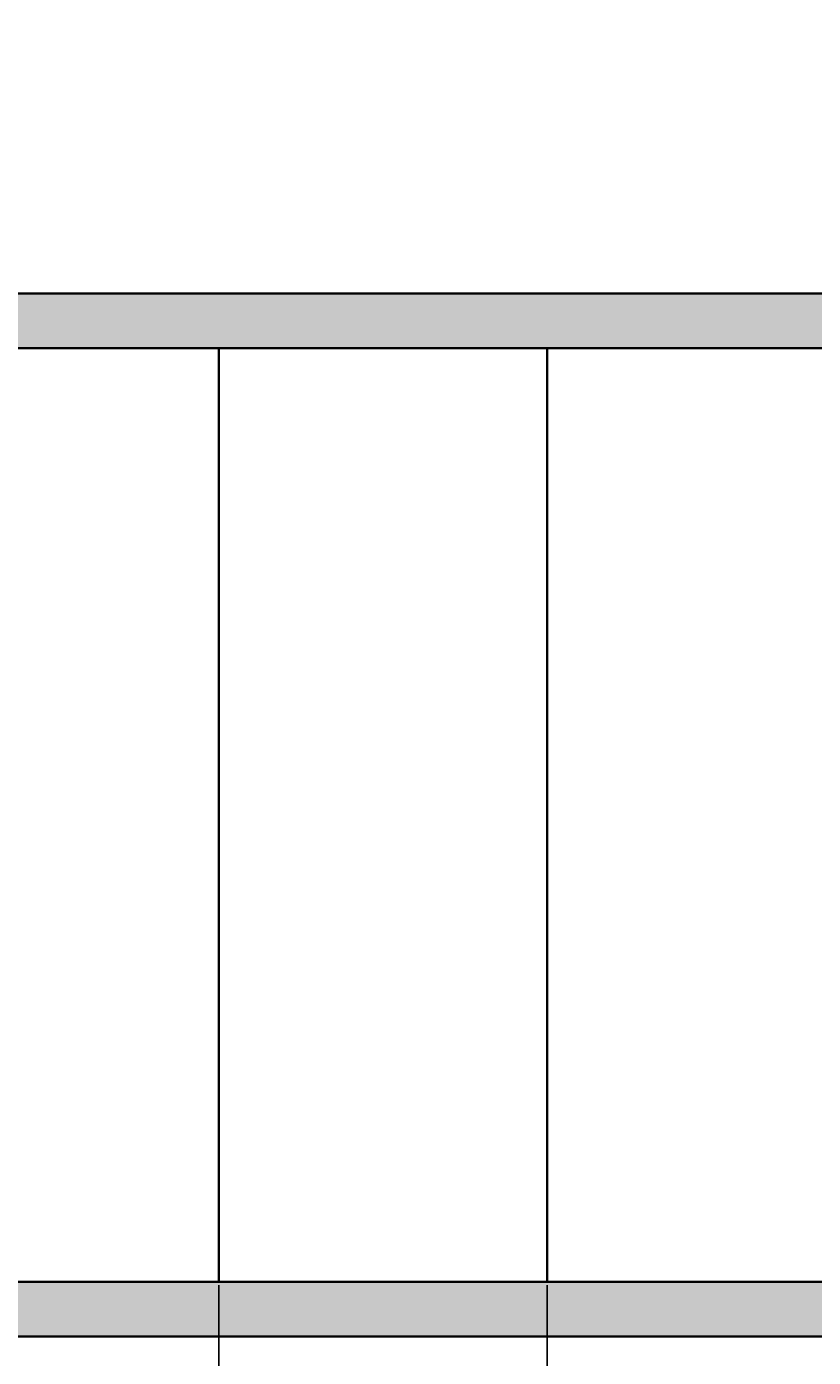
# Model space of a CAD drawing. Units: millimetres. Extents: x -22994 to 29398, y -19990 to 20176.
# Tile 35 of 135: x 169 to 183, y 30 to 54. Entities that reach past the tile are written whole.
import ezdxf

# ---------------------------------------------------------------- set-up
doc = ezdxf.new("R2010")
doc.units = ezdxf.units.MM
doc.header["$MEASUREMENT"] = 0
for name, color, linetype, lineweight in [('M-DIMS', 2, 'Continuous', 18), ('M-EQPM-PATT', 7, 'Continuous', 18), ('M-PIPE', 7, 'Continuous', 35)]:
    doc.layers.add(name, color=color, linetype=linetype, lineweight=lineweight)
doc.styles.get("Standard").update_dxf_attribs({"font": 'arial.ttf'})
doc.dimstyles.get("Standard").update_dxf_attribs({"dimtxt": 0.18, "dimasz": 10000, "dimexe": 0.18, "dimexo": 0.0625, "dimgap": 0.09, "dimtad": 0, "dimtih": 1, "dimtoh": 1, "dimdec": 0, "dimzin": 0, "dimdsep": 46, "dimtxsty": 'Standard', "dimcen": 0.09, "dimadec": 0, "dimazin": 0, "dimtfac": 1, "dimtdec": 0, "dimtofl": 0, "dimtmove": 0, "dimatfit": 3, "dimfxl": 1, "dimtolj": 1, "dimtzin": 0, "dimlwd": 30, "dimarcsym": 0})

# ---------------------------------------------------------------- blocks, each defined once
blk = doc.blocks.new('*D2')
at = {"layer": 'Defpoints', "color": 0, "transparency": 16777216}
for p in [(6.677, 10.271), (290.852, 10.271), (290.852, -5.079)]:
    blk.add_point(p, dxfattribs=at)
at = {"layer": 'M-DIMS', "color": 0, "lineweight": -2, "transparency": 16777216}
for p, q in [((6.677, 10.209), (6.677, -5.259)), ((290.852, 10.209), (290.852, -5.259))]:
    blk.add_line(p, q, dxfattribs=at)
at = {"layer": 'M-DIMS', "color": 0, "lineweight": 30, "transparency": 16777216}
for p, q in [((-9993.323, -5.079), (-19993.323, -5.079)), ((10290.852, -5.079), (20290.852, -5.079))]:
    blk.add_line(p, q, dxfattribs=at)
at = {"layer": 'M-DIMS', "color": 0, "transparency": 16777216}
for points in [[(-9993.323, 1661.588), (-9993.323, -1671.745), (6.677, -5.079)], [(10290.852, 1661.588), (10290.852, -1671.745), (290.852, -5.079)]]:
    blk.add_solid(points, dxfattribs=at)
at = {"layer": 'M-DIMS', "color": 0, "transparency": 16777216, "insert": (148.765, -5.079), "char_height": 0.18, "attachment_point": 5}
blk.add_mtext('\\A1;284.2', dxfattribs=at)
blk = doc.blocks.new('*D3')
at = {"layer": 'Defpoints', "color": 0, "transparency": 16777216}
for p in [(110.265, 204.165), (110.265, 176.366), (95.833, 127.967)]:
    blk.add_point(p, dxfattribs=at)
at = {"layer": 'M-DIMS', "color": 0, "lineweight": -2, "transparency": 16777216}
for p, q in [((95.833, 128.03), (95.833, 204.345)), ((110.265, 176.429), (110.265, 204.345))]:
    blk.add_line(p, q, dxfattribs=at)
at = {"layer": 'M-DIMS', "color": 0, "lineweight": 30, "transparency": 16777216}
for p, q in [((-9904.167, 204.165), (-19904.167, 204.165)), ((10110.265, 204.165), (20110.265, 204.165))]:
    blk.add_line(p, q, dxfattribs=at)
at = {"layer": 'M-DIMS', "color": 0, "transparency": 16777216}
for points in [[(-9904.167, 1870.832), (-9904.167, -1462.501), (95.833, 204.165)], [(10110.265, 1870.832), (10110.265, -1462.501), (110.265, 204.165)]]:
    blk.add_solid(points, dxfattribs=at)
at = {"layer": 'M-DIMS', "color": 0, "transparency": 16777216, "insert": (103.049, 204.165), "char_height": 0.18, "attachment_point": 5}
blk.add_mtext('\\A1;14.432', dxfattribs=at)
blk = doc.blocks.new('*D4')
at = {"layer": 'Defpoints', "color": 0, "transparency": 16777216}
for p in [(116.265, 204.165), (110.265, 176.366), (116.265, 176.366)]:
    blk.add_point(p, dxfattribs=at)
at = {"layer": 'M-DIMS', "color": 0, "lineweight": -2, "transparency": 16777216}
for p, q in [((110.265, 176.429), (110.265, 204.345)), ((116.265, 176.429), (116.265, 204.345))]:
    blk.add_line(p, q, dxfattribs=at)
at = {"layer": 'M-DIMS', "color": 0, "lineweight": 30, "transparency": 16777216}
for p, q in [((-9889.735, 204.165), (-19889.735, 204.165)), ((10116.265, 204.165), (20116.265, 204.165))]:
    blk.add_line(p, q, dxfattribs=at)
at = {"layer": 'M-DIMS', "color": 0, "transparency": 16777216}
for points in [[(-9889.735, 1870.832), (-9889.735, -1462.501), (110.265, 204.165)], [(10116.265, 1870.832), (10116.265, -1462.501), (116.265, 204.165)]]:
    blk.add_solid(points, dxfattribs=at)
at = {"layer": 'M-DIMS', "color": 0, "transparency": 16777216, "insert": (113.265, 204.165), "char_height": 0.18, "attachment_point": 5}
blk.add_mtext('\\A1;6', dxfattribs=at)
blk = doc.blocks.new('*D5')
at = {"layer": 'Defpoints', "color": 0, "transparency": 16777216}
for p in [(181.265, 204.165), (116.265, 176.366), (181.265, 176.366)]:
    blk.add_point(p, dxfattribs=at)
at = {"layer": 'M-DIMS', "color": 0, "lineweight": -2, "transparency": 16777216}
for p, q in [((116.265, 176.429), (116.265, 204.345)), ((181.265, 176.429), (181.265, 204.345))]:
    blk.add_line(p, q, dxfattribs=at)
at = {"layer": 'M-DIMS', "color": 0, "lineweight": 30, "transparency": 16777216}
for p, q in [((-9883.735, 204.165), (-19883.735, 204.165)), ((10181.265, 204.165), (20181.265, 204.165))]:
    blk.add_line(p, q, dxfattribs=at)
at = {"layer": 'M-DIMS', "color": 0, "transparency": 16777216}
for points in [[(-9883.735, 1870.832), (-9883.735, -1462.501), (116.265, 204.165)], [(10181.265, 1870.832), (10181.265, -1462.501), (181.265, 204.165)]]:
    blk.add_solid(points, dxfattribs=at)
at = {"layer": 'M-DIMS', "color": 0, "transparency": 16777216, "insert": (148.765, 204.165), "char_height": 0.18, "attachment_point": 5}
blk.add_mtext('\\A1;65', dxfattribs=at)
blk = doc.blocks.new('*D6')
at = {"layer": 'Defpoints', "color": 0, "transparency": 16777216}
for p in [(187.265, 204.165), (181.265, 176.366), (187.265, 176.366)]:
    blk.add_point(p, dxfattribs=at)
at = {"layer": 'M-DIMS', "color": 0, "lineweight": -2, "transparency": 16777216}
for p, q in [((181.265, 176.429), (181.265, 204.345)), ((187.265, 176.429), (187.265, 204.345))]:
    blk.add_line(p, q, dxfattribs=at)
at = {"layer": 'M-DIMS', "color": 0, "lineweight": 30, "transparency": 16777216}
for p, q in [((-9818.735, 204.165), (-19818.735, 204.165)), ((10187.265, 204.165), (20187.265, 204.165))]:
    blk.add_line(p, q, dxfattribs=at)
at = {"layer": 'M-DIMS', "color": 0, "transparency": 16777216}
for points in [[(-9818.735, 1870.832), (-9818.735, -1462.501), (181.265, 204.165)], [(10187.265, 1870.832), (10187.265, -1462.501), (187.265, 204.165)]]:
    blk.add_solid(points, dxfattribs=at)
at = {"layer": 'M-DIMS', "color": 0, "transparency": 16777216, "insert": (184.265, 204.165), "char_height": 0.18, "attachment_point": 5}
blk.add_mtext('\\A1;6', dxfattribs=at)
blk = doc.blocks.new('*D7')
at = {"layer": 'Defpoints', "color": 0, "transparency": 16777216}
for p in [(201.697, 204.165), (187.265, 176.366), (201.697, 127.967)]:
    blk.add_point(p, dxfattribs=at)
at = {"layer": 'M-DIMS', "color": 0, "lineweight": -2, "transparency": 16777216}
for p, q in [((187.265, 176.429), (187.265, 204.345)), ((201.697, 128.03), (201.697, 204.345))]:
    blk.add_line(p, q, dxfattribs=at)
at = {"layer": 'M-DIMS', "color": 0, "lineweight": 30, "transparency": 16777216}
for p, q in [((-9812.735, 204.165), (-19812.735, 204.165)), ((10201.697, 204.165), (20201.697, 204.165))]:
    blk.add_line(p, q, dxfattribs=at)
at = {"layer": 'M-DIMS', "color": 0, "transparency": 16777216}
for points in [[(-9812.735, 1870.832), (-9812.735, -1462.501), (187.265, 204.165)], [(10201.697, 1870.832), (10201.697, -1462.501), (201.697, 204.165)]]:
    blk.add_solid(points, dxfattribs=at)
at = {"layer": 'M-DIMS', "color": 0, "transparency": 16777216, "insert": (194.481, 204.165), "char_height": 0.18, "attachment_point": 5}
blk.add_mtext('\\A1;14.432', dxfattribs=at)
blk = doc.blocks.new('*D8')
at = {"layer": 'Defpoints', "color": 0, "transparency": 16777216}
for p in [(227.648, 204.165), (227.648, 146.73), (201.697, 127.967)]:
    blk.add_point(p, dxfattribs=at)
at = {"layer": 'M-DIMS', "color": 0, "lineweight": -2, "transparency": 16777216}
for p, q in [((201.697, 128.03), (201.697, 204.345)), ((227.648, 146.792), (227.648, 204.345))]:
    blk.add_line(p, q, dxfattribs=at)
at = {"layer": 'M-DIMS', "color": 0, "lineweight": 30, "transparency": 16777216}
for p, q in [((-9798.303, 204.165), (-19798.303, 204.165)), ((10227.648, 204.165), (20227.648, 204.165))]:
    blk.add_line(p, q, dxfattribs=at)
at = {"layer": 'M-DIMS', "color": 0, "transparency": 16777216}
for points in [[(-9798.303, 1870.832), (-9798.303, -1462.501), (201.697, 204.165)], [(10227.648, 1870.832), (10227.648, -1462.501), (227.648, 204.165)]]:
    blk.add_solid(points, dxfattribs=at)
at = {"layer": 'M-DIMS', "color": 0, "transparency": 16777216, "insert": (214.673, 204.165), "char_height": 0.18, "attachment_point": 5}
blk.add_mtext('\\A1;25.95', dxfattribs=at)
blk = doc.blocks.new('*D9')
at = {"layer": 'Defpoints', "color": 0, "transparency": 16777216}
for p in [(187.265, 176.366), (306.202, 176.366), (290.852, 10.271)]:
    blk.add_point(p, dxfattribs=at)
at = {"layer": 'M-DIMS', "color": 0, "lineweight": 30, "transparency": 16777216}
for p, q in [((306.202, 10176.366), (306.202, 20176.366)), ((306.202, -9989.729), (306.202, -19989.729))]:
    blk.add_line(p, q, dxfattribs=at)
at = {"layer": 'M-DIMS', "color": 0, "lineweight": -2, "transparency": 16777216}
for p, q in [((187.327, 176.366), (306.382, 176.366)), ((290.915, 10.271), (306.382, 10.271))]:
    blk.add_line(p, q, dxfattribs=at)
at = {"layer": 'M-DIMS', "color": 0, "transparency": 16777216}
for points in [[(-1360.465, 10176.366), (1972.869, 10176.366), (306.202, 176.366)], [(-1360.465, -9989.729), (1972.869, -9989.729), (306.202, 10.271)]]:
    blk.add_solid(points, dxfattribs=at)
at = {"layer": 'M-DIMS', "color": 0, "transparency": 16777216, "insert": (306.202, 93.319), "char_height": 0.18, "attachment_point": 5}
blk.add_mtext('\\A1;166.1', dxfattribs=at)
blk = doc.blocks.new('*D10')
at = {"layer": 'Defpoints', "color": 0, "transparency": 16777216}
for p in [(125.65, 136.071), (133.346, 136.071), (133.346, -5.079)]:
    blk.add_point(p, dxfattribs=at)
at = {"layer": 'M-DIMS', "color": 0, "lineweight": -2, "transparency": 16777216}
for p, q in [((125.65, 136.009), (125.65, -5.259)), ((133.346, 136.009), (133.346, -5.259))]:
    blk.add_line(p, q, dxfattribs=at)
at = {"layer": 'M-DIMS', "color": 0, "lineweight": 30, "transparency": 16777216}
for p, q in [((-9874.35, -5.079), (-19874.35, -5.079)), ((10133.346, -5.079), (20133.346, -5.079))]:
    blk.add_line(p, q, dxfattribs=at)
at = {"layer": 'M-DIMS', "color": 0, "transparency": 16777216}
for points in [[(-9874.35, 1661.588), (-9874.35, -1671.745), (125.65, -5.079)], [(10133.346, 1661.588), (10133.346, -1671.745), (133.346, -5.079)]]:
    blk.add_solid(points, dxfattribs=at)
at = {"layer": 'M-DIMS', "color": 0, "transparency": 16777216, "insert": (129.498, -5.079), "char_height": 0.18, "attachment_point": 5}
blk.add_mtext('\\A1;7.696', dxfattribs=at)
blk = doc.blocks.new('*D11')
at = {"layer": 'Defpoints', "color": 0, "transparency": 16777216}
for p in [(133.346, 136.071), (135.65, 136.071), (135.65, -5.079)]:
    blk.add_point(p, dxfattribs=at)
at = {"layer": 'M-DIMS', "color": 0, "lineweight": -2, "transparency": 16777216}
for p, q in [((133.346, 136.009), (133.346, -5.259)), ((135.65, 136.009), (135.65, -5.259))]:
    blk.add_line(p, q, dxfattribs=at)
at = {"layer": 'M-DIMS', "color": 0, "lineweight": 30, "transparency": 16777216}
for p, q in [((-9866.654, -5.079), (-19866.654, -5.079)), ((10135.65, -5.079), (20135.65, -5.079))]:
    blk.add_line(p, q, dxfattribs=at)
at = {"layer": 'M-DIMS', "color": 0, "transparency": 16777216}
for points in [[(-9866.654, 1661.588), (-9866.654, -1671.745), (133.346, -5.079)], [(10135.65, 1661.588), (10135.65, -1671.745), (135.65, -5.079)]]:
    blk.add_solid(points, dxfattribs=at)
at = {"layer": 'M-DIMS', "color": 0, "transparency": 16777216, "insert": (134.498, -5.079), "char_height": 0.18, "attachment_point": 5}
blk.add_mtext('\\A1;2.304', dxfattribs=at)
blk = doc.blocks.new('*D12')
at = {"layer": 'Defpoints', "color": 0, "transparency": 16777216}
for p in [(135.65, 136.071), (145.65, 136.071), (145.65, -5.079)]:
    blk.add_point(p, dxfattribs=at)
at = {"layer": 'M-DIMS', "color": 0, "lineweight": -2, "transparency": 16777216}
for p, q in [((135.65, 136.009), (135.65, -5.259)), ((145.65, 136.009), (145.65, -5.259))]:
    blk.add_line(p, q, dxfattribs=at)
at = {"layer": 'M-DIMS', "color": 0, "lineweight": 30, "transparency": 16777216}
for p, q in [((-9864.35, -5.079), (-19864.35, -5.079)), ((10145.65, -5.079), (20145.65, -5.079))]:
    blk.add_line(p, q, dxfattribs=at)
at = {"layer": 'M-DIMS', "color": 0, "transparency": 16777216}
for points in [[(-9864.35, 1661.588), (-9864.35, -1671.745), (135.65, -5.079)], [(10145.65, 1661.588), (10145.65, -1671.745), (145.65, -5.079)]]:
    blk.add_solid(points, dxfattribs=at)
at = {"layer": 'M-DIMS', "color": 0, "transparency": 16777216, "insert": (140.65, -5.079), "char_height": 0.18, "attachment_point": 5}
blk.add_mtext('\\A1;10', dxfattribs=at)
blk = doc.blocks.new('*D13')
at = {"layer": 'Defpoints', "color": 0, "transparency": 16777216}
for p in [(145.65, 136.071), (155.65, 136.071), (155.65, -5.079)]:
    blk.add_point(p, dxfattribs=at)
at = {"layer": 'M-DIMS', "color": 0, "lineweight": -2, "transparency": 16777216}
for p, q in [((145.65, 136.009), (145.65, -5.259)), ((155.65, 136.009), (155.65, -5.259))]:
    blk.add_line(p, q, dxfattribs=at)
at = {"layer": 'M-DIMS', "color": 0, "lineweight": 30, "transparency": 16777216}
for p, q in [((-9854.35, -5.079), (-19854.35, -5.079)), ((10155.65, -5.079), (20155.65, -5.079))]:
    blk.add_line(p, q, dxfattribs=at)
at = {"layer": 'M-DIMS', "color": 0, "transparency": 16777216}
for points in [[(-9854.35, 1661.588), (-9854.35, -1671.745), (145.65, -5.079)], [(10155.65, 1661.588), (10155.65, -1671.745), (155.65, -5.079)]]:
    blk.add_solid(points, dxfattribs=at)
at = {"layer": 'M-DIMS', "color": 0, "transparency": 16777216, "insert": (150.65, -5.079), "char_height": 0.18, "attachment_point": 5}
blk.add_mtext('\\A1;10', dxfattribs=at)
blk = doc.blocks.new('*D14')
at = {"layer": 'Defpoints', "color": 0, "transparency": 16777216}
for p in [(155.65, 136.071), (165.65, 136.071), (165.65, -5.079)]:
    blk.add_point(p, dxfattribs=at)
at = {"layer": 'M-DIMS', "color": 0, "lineweight": -2, "transparency": 16777216}
for p, q in [((155.65, 136.009), (155.65, -5.259)), ((165.65, 136.009), (165.65, -5.259))]:
    blk.add_line(p, q, dxfattribs=at)
at = {"layer": 'M-DIMS', "color": 0, "lineweight": 30, "transparency": 16777216}
for p, q in [((-9844.35, -5.079), (-19844.35, -5.079)), ((10165.65, -5.079), (20165.65, -5.079))]:
    blk.add_line(p, q, dxfattribs=at)
at = {"layer": 'M-DIMS', "color": 0, "transparency": 16777216}
for points in [[(-9844.35, 1661.588), (-9844.35, -1671.745), (155.65, -5.079)], [(10165.65, 1661.588), (10165.65, -1671.745), (165.65, -5.079)]]:
    blk.add_solid(points, dxfattribs=at)
at = {"layer": 'M-DIMS', "color": 0, "transparency": 16777216, "insert": (160.65, -5.079), "char_height": 0.18, "attachment_point": 5}
blk.add_mtext('\\A1;10', dxfattribs=at)
blk = doc.blocks.new('*D15')
at = {"layer": 'Defpoints', "color": 0, "transparency": 16777216}
for p in [(173.346, 154.788), (173.346, 136.071), (306.202, 136.071)]:
    blk.add_point(p, dxfattribs=at)
at = {"layer": 'M-DIMS', "color": 0, "lineweight": 30, "transparency": 16777216}
for p, q in [((306.202, 10154.788), (306.202, 20154.788)), ((306.202, -9863.929), (306.202, -19863.929))]:
    blk.add_line(p, q, dxfattribs=at)
at = {"layer": 'M-DIMS', "color": 0, "lineweight": -2, "transparency": 16777216}
for p, q in [((173.408, 154.788), (306.382, 154.788)), ((173.408, 136.071), (306.382, 136.071))]:
    blk.add_line(p, q, dxfattribs=at)
at = {"layer": 'M-DIMS', "color": 0, "transparency": 16777216}
for points in [[(-1360.465, 10154.788), (1972.869, 10154.788), (306.202, 154.788)], [(-1360.465, -9863.929), (1972.869, -9863.929), (306.202, 136.071)]]:
    blk.add_solid(points, dxfattribs=at)
at = {"layer": 'M-DIMS', "color": 0, "transparency": 16777216, "insert": (306.202, 145.43), "char_height": 0.18, "attachment_point": 5}
blk.add_mtext('\\A1;18.717', dxfattribs=at)
blk = doc.blocks.new('*D16')
at = {"layer": 'Defpoints', "color": 0, "transparency": 16777216}
for p in [(120.17, 204.165), (110.466, 48.035), (120.17, 48.035)]:
    blk.add_point(p, dxfattribs=at)
at = {"layer": 'M-DIMS', "color": 0, "lineweight": -2, "transparency": 16777216}
for p, q in [((110.466, 48.097), (110.466, 204.345)), ((120.17, 48.097), (120.17, 204.345))]:
    blk.add_line(p, q, dxfattribs=at)
at = {"layer": 'M-DIMS', "color": 0, "lineweight": 30, "transparency": 16777216}
for p, q in [((-9889.534, 204.165), (-19889.534, 204.165)), ((10120.17, 204.165), (20120.17, 204.165))]:
    blk.add_line(p, q, dxfattribs=at)
at = {"layer": 'M-DIMS', "color": 0, "transparency": 16777216}
for points in [[(-9889.534, 1870.832), (-9889.534, -1462.501), (110.466, 204.165)], [(10120.17, 1870.832), (10120.17, -1462.501), (120.17, 204.165)]]:
    blk.add_solid(points, dxfattribs=at)
at = {"layer": 'M-DIMS', "color": 0, "transparency": 16777216, "insert": (115.318, 204.165), "char_height": 0.18, "attachment_point": 5}
blk.add_mtext('\\A1;9.704', dxfattribs=at)
blk = doc.blocks.new('*D17')
at = {"layer": 'Defpoints', "color": 0, "transparency": 16777216}
for p in [(126.17, 204.165), (120.17, 48.035), (126.17, 48.035)]:
    blk.add_point(p, dxfattribs=at)
at = {"layer": 'M-DIMS', "color": 0, "lineweight": -2, "transparency": 16777216}
for p, q in [((120.17, 48.097), (120.17, 204.345)), ((126.17, 48.097), (126.17, 204.345))]:
    blk.add_line(p, q, dxfattribs=at)
at = {"layer": 'M-DIMS', "color": 0, "lineweight": 30, "transparency": 16777216}
for p, q in [((-9879.83, 204.165), (-19879.83, 204.165)), ((10126.17, 204.165), (20126.17, 204.165))]:
    blk.add_line(p, q, dxfattribs=at)
at = {"layer": 'M-DIMS', "color": 0, "transparency": 16777216}
for points in [[(-9879.83, 1870.832), (-9879.83, -1462.501), (120.17, 204.165)], [(10126.17, 1870.832), (10126.17, -1462.501), (126.17, 204.165)]]:
    blk.add_solid(points, dxfattribs=at)
at = {"layer": 'M-DIMS', "color": 0, "transparency": 16777216, "insert": (123.17, 204.165), "char_height": 0.18, "attachment_point": 5}
blk.add_mtext('\\A1;6', dxfattribs=at)
blk = doc.blocks.new('*D18')
at = {"layer": 'Defpoints', "color": 0, "transparency": 16777216}
for p in [(132.17, 204.165), (126.17, 48.035), (132.17, 48.035)]:
    blk.add_point(p, dxfattribs=at)
at = {"layer": 'M-DIMS', "color": 0, "lineweight": -2, "transparency": 16777216}
for p, q in [((126.17, 48.097), (126.17, 204.345)), ((132.17, 48.097), (132.17, 204.345))]:
    blk.add_line(p, q, dxfattribs=at)
at = {"layer": 'M-DIMS', "color": 0, "lineweight": 30, "transparency": 16777216}
for p, q in [((-9873.83, 204.165), (-19873.83, 204.165)), ((10132.17, 204.165), (20132.17, 204.165))]:
    blk.add_line(p, q, dxfattribs=at)
at = {"layer": 'M-DIMS', "color": 0, "transparency": 16777216}
for points in [[(-9873.83, 1870.832), (-9873.83, -1462.501), (126.17, 204.165)], [(10132.17, 1870.832), (10132.17, -1462.501), (132.17, 204.165)]]:
    blk.add_solid(points, dxfattribs=at)
at = {"layer": 'M-DIMS', "color": 0, "transparency": 16777216, "insert": (129.17, 204.165), "char_height": 0.18, "attachment_point": 5}
blk.add_mtext('\\A1;6', dxfattribs=at)
blk = doc.blocks.new('*D19')
at = {"layer": 'Defpoints', "color": 0, "transparency": 16777216}
for p in [(138.17, 204.165), (132.17, 48.035), (138.17, 48.035)]:
    blk.add_point(p, dxfattribs=at)
at = {"layer": 'M-DIMS', "color": 0, "lineweight": -2, "transparency": 16777216}
for p, q in [((132.17, 48.097), (132.17, 204.345)), ((138.17, 48.097), (138.17, 204.345))]:
    blk.add_line(p, q, dxfattribs=at)
at = {"layer": 'M-DIMS', "color": 0, "lineweight": 30, "transparency": 16777216}
for p, q in [((-9867.83, 204.165), (-19867.83, 204.165)), ((10138.17, 204.165), (20138.17, 204.165))]:
    blk.add_line(p, q, dxfattribs=at)
at = {"layer": 'M-DIMS', "color": 0, "transparency": 16777216}
for points in [[(-9867.83, 1870.832), (-9867.83, -1462.501), (132.17, 204.165)], [(10138.17, 1870.832), (10138.17, -1462.501), (138.17, 204.165)]]:
    blk.add_solid(points, dxfattribs=at)
at = {"layer": 'M-DIMS', "color": 0, "transparency": 16777216, "insert": (135.17, 204.165), "char_height": 0.18, "attachment_point": 5}
blk.add_mtext('\\A1;6', dxfattribs=at)
blk = doc.blocks.new('*D20')
at = {"layer": 'Defpoints', "color": 0, "transparency": 16777216}
for p in [(144.17, 204.165), (138.17, 48.035), (144.17, 48.035)]:
    blk.add_point(p, dxfattribs=at)
at = {"layer": 'M-DIMS', "color": 0, "lineweight": -2, "transparency": 16777216}
for p, q in [((138.17, 48.097), (138.17, 204.345)), ((144.17, 48.097), (144.17, 204.345))]:
    blk.add_line(p, q, dxfattribs=at)
at = {"layer": 'M-DIMS', "color": 0, "lineweight": 30, "transparency": 16777216}
for p, q in [((-9861.83, 204.165), (-19861.83, 204.165)), ((10144.17, 204.165), (20144.17, 204.165))]:
    blk.add_line(p, q, dxfattribs=at)
at = {"layer": 'M-DIMS', "color": 0, "transparency": 16777216}
for points in [[(-9861.83, 1870.832), (-9861.83, -1462.501), (138.17, 204.165)], [(10144.17, 1870.832), (10144.17, -1462.501), (144.17, 204.165)]]:
    blk.add_solid(points, dxfattribs=at)
at = {"layer": 'M-DIMS', "color": 0, "transparency": 16777216, "insert": (141.17, 204.165), "char_height": 0.18, "attachment_point": 5}
blk.add_mtext('\\A1;6', dxfattribs=at)
blk = doc.blocks.new('*D21')
at = {"layer": 'Defpoints', "color": 0, "transparency": 16777216}
for p in [(149.116, 204.165), (144.17, 48.035), (149.116, 48.035)]:
    blk.add_point(p, dxfattribs=at)
at = {"layer": 'M-DIMS', "color": 0, "lineweight": -2, "transparency": 16777216}
for p, q in [((144.17, 48.097), (144.17, 204.345)), ((149.116, 48.097), (149.116, 204.345))]:
    blk.add_line(p, q, dxfattribs=at)
at = {"layer": 'M-DIMS', "color": 0, "lineweight": 30, "transparency": 16777216}
for p, q in [((-9855.83, 204.165), (-19855.83, 204.165)), ((10149.116, 204.165), (20149.116, 204.165))]:
    blk.add_line(p, q, dxfattribs=at)
at = {"layer": 'M-DIMS', "color": 0, "transparency": 16777216}
for points in [[(-9855.83, 1870.832), (-9855.83, -1462.501), (144.17, 204.165)], [(10149.116, 1870.832), (10149.116, -1462.501), (149.116, 204.165)]]:
    blk.add_solid(points, dxfattribs=at)
at = {"layer": 'M-DIMS', "color": 0, "transparency": 16777216, "insert": (146.643, 204.165), "char_height": 0.18, "attachment_point": 5}
blk.add_mtext('\\A1;4.945', dxfattribs=at)
blk = doc.blocks.new('*D22')
at = {"layer": 'Defpoints', "color": 0, "transparency": 16777216}
for p in [(149.116, 30.99), (155.116, 30.99), (155.116, -5.079)]:
    blk.add_point(p, dxfattribs=at)
at = {"layer": 'M-DIMS', "color": 0, "lineweight": -2, "transparency": 16777216}
for p, q in [((149.116, 30.927), (149.116, -5.259)), ((155.116, 30.927), (155.116, -5.259))]:
    blk.add_line(p, q, dxfattribs=at)
at = {"layer": 'M-DIMS', "color": 0, "lineweight": 30, "transparency": 16777216}
for p, q in [((-9850.884, -5.079), (-19850.884, -5.079)), ((10155.116, -5.079), (20155.116, -5.079))]:
    blk.add_line(p, q, dxfattribs=at)
at = {"layer": 'M-DIMS', "color": 0, "transparency": 16777216}
for points in [[(-9850.884, 1661.588), (-9850.884, -1671.745), (149.116, -5.079)], [(10155.116, 1661.588), (10155.116, -1671.745), (155.116, -5.079)]]:
    blk.add_solid(points, dxfattribs=at)
at = {"layer": 'M-DIMS', "color": 0, "transparency": 16777216, "insert": (152.116, -5.079), "char_height": 0.18, "attachment_point": 5}
blk.add_mtext('\\A1;6', dxfattribs=at)
blk = doc.blocks.new('*D23')
at = {"layer": 'Defpoints', "color": 0, "transparency": 16777216}
for p in [(155.116, 30.99), (161.116, 30.99), (161.116, -5.079)]:
    blk.add_point(p, dxfattribs=at)
at = {"layer": 'M-DIMS', "color": 0, "lineweight": -2, "transparency": 16777216}
for p, q in [((155.116, 30.927), (155.116, -5.259)), ((161.116, 30.927), (161.116, -5.259))]:
    blk.add_line(p, q, dxfattribs=at)
at = {"layer": 'M-DIMS', "color": 0, "lineweight": 30, "transparency": 16777216}
for p, q in [((-9844.884, -5.079), (-19844.884, -5.079)), ((10161.116, -5.079), (20161.116, -5.079))]:
    blk.add_line(p, q, dxfattribs=at)
at = {"layer": 'M-DIMS', "color": 0, "transparency": 16777216}
for points in [[(-9844.884, 1661.588), (-9844.884, -1671.745), (155.116, -5.079)], [(10161.116, 1661.588), (10161.116, -1671.745), (161.116, -5.079)]]:
    blk.add_solid(points, dxfattribs=at)
at = {"layer": 'M-DIMS', "color": 0, "transparency": 16777216, "insert": (158.116, -5.079), "char_height": 0.18, "attachment_point": 5}
blk.add_mtext('\\A1;6', dxfattribs=at)
blk = doc.blocks.new('*D24')
at = {"layer": 'Defpoints', "color": 0, "transparency": 16777216}
for p in [(161.116, 30.99), (166.439, 30.99), (166.439, -5.079)]:
    blk.add_point(p, dxfattribs=at)
at = {"layer": 'M-DIMS', "color": 0, "lineweight": -2, "transparency": 16777216}
for p, q in [((161.116, 30.927), (161.116, -5.259)), ((166.439, 30.927), (166.439, -5.259))]:
    blk.add_line(p, q, dxfattribs=at)
at = {"layer": 'M-DIMS', "color": 0, "lineweight": 30, "transparency": 16777216}
for p, q in [((-9838.884, -5.079), (-19838.884, -5.079)), ((10166.439, -5.079), (20166.439, -5.079))]:
    blk.add_line(p, q, dxfattribs=at)
at = {"layer": 'M-DIMS', "color": 0, "transparency": 16777216}
for points in [[(-9838.884, 1661.588), (-9838.884, -1671.745), (161.116, -5.079)], [(10166.439, 1661.588), (10166.439, -1671.745), (166.439, -5.079)]]:
    blk.add_solid(points, dxfattribs=at)
at = {"layer": 'M-DIMS', "color": 0, "transparency": 16777216, "insert": (163.777, -5.079), "char_height": 0.18, "attachment_point": 5}
blk.add_mtext('\\A1;5.323', dxfattribs=at)
blk = doc.blocks.new('*D25')
at = {"layer": 'Defpoints', "color": 0, "transparency": 16777216}
for p in [(166.439, 30.99), (172.439, 30.99), (172.439, -5.079)]:
    blk.add_point(p, dxfattribs=at)
at = {"layer": 'M-DIMS', "color": 0, "lineweight": -2, "transparency": 16777216}
for p, q in [((166.439, 30.927), (166.439, -5.259)), ((172.439, 30.927), (172.439, -5.259))]:
    blk.add_line(p, q, dxfattribs=at)
at = {"layer": 'M-DIMS', "color": 0, "lineweight": 30, "transparency": 16777216}
for p, q in [((-9833.561, -5.079), (-19833.561, -5.079)), ((10172.439, -5.079), (20172.439, -5.079))]:
    blk.add_line(p, q, dxfattribs=at)
at = {"layer": 'M-DIMS', "color": 0, "transparency": 16777216}
for points in [[(-9833.561, 1661.588), (-9833.561, -1671.745), (166.439, -5.079)], [(10172.439, 1661.588), (10172.439, -1671.745), (172.439, -5.079)]]:
    blk.add_solid(points, dxfattribs=at)
at = {"layer": 'M-DIMS', "color": 0, "transparency": 16777216, "insert": (169.439, -5.079), "char_height": 0.18, "attachment_point": 5}
blk.add_mtext('\\A1;6', dxfattribs=at)
blk = doc.blocks.new('*D26')
at = {"layer": 'Defpoints', "color": 0, "transparency": 16777216}
for p in [(172.439, 30.99), (178.439, 30.99), (178.439, -5.079)]:
    blk.add_point(p, dxfattribs=at)
at = {"layer": 'M-DIMS', "color": 0, "lineweight": -2, "transparency": 16777216}
for p, q in [((172.439, 30.927), (172.439, -5.259)), ((178.439, 30.927), (178.439, -5.259))]:
    blk.add_line(p, q, dxfattribs=at)
at = {"layer": 'M-DIMS', "color": 0, "lineweight": 30, "transparency": 16777216}
for p, q in [((-9827.561, -5.079), (-19827.561, -5.079)), ((10178.439, -5.079), (20178.439, -5.079))]:
    blk.add_line(p, q, dxfattribs=at)
at = {"layer": 'M-DIMS', "color": 0, "transparency": 16777216}
for points in [[(-9827.561, 1661.588), (-9827.561, -1671.745), (172.439, -5.079)], [(10178.439, 1661.588), (10178.439, -1671.745), (178.439, -5.079)]]:
    blk.add_solid(points, dxfattribs=at)
at = {"layer": 'M-DIMS', "color": 0, "transparency": 16777216, "insert": (175.439, -5.079), "char_height": 0.18, "attachment_point": 5}
blk.add_mtext('\\A1;6', dxfattribs=at)
blk = doc.blocks.new('*D27')
at = {"layer": 'Defpoints', "color": 0, "transparency": 16777216}
for p in [(178.439, 30.99), (188.117, 30.99), (188.117, -5.079)]:
    blk.add_point(p, dxfattribs=at)
at = {"layer": 'M-DIMS', "color": 0, "lineweight": -2, "transparency": 16777216}
for p, q in [((178.439, 30.927), (178.439, -5.259)), ((188.117, 30.927), (188.117, -5.259))]:
    blk.add_line(p, q, dxfattribs=at)
at = {"layer": 'M-DIMS', "color": 0, "lineweight": 30, "transparency": 16777216}
for p, q in [((-9821.561, -5.079), (-19821.561, -5.079)), ((10188.117, -5.079), (20188.117, -5.079))]:
    blk.add_line(p, q, dxfattribs=at)
at = {"layer": 'M-DIMS', "color": 0, "transparency": 16777216}
for points in [[(-9821.561, 1661.588), (-9821.561, -1671.745), (178.439, -5.079)], [(10188.117, 1661.588), (10188.117, -1671.745), (188.117, -5.079)]]:
    blk.add_solid(points, dxfattribs=at)
at = {"layer": 'M-DIMS', "color": 0, "transparency": 16777216, "insert": (183.278, -5.079), "char_height": 0.18, "attachment_point": 5}
blk.add_mtext('\\A1;9.679', dxfattribs=at)
blk = doc.blocks.new('*D28')
at = {"layer": 'Defpoints', "color": 0, "transparency": 16777216}
for p in [(188.117, 48.035), (306.202, 48.035), (188.117, 30.99)]:
    blk.add_point(p, dxfattribs=at)
at = {"layer": 'M-DIMS', "color": 0, "lineweight": 30, "transparency": 16777216}
for p, q in [((306.202, 10048.035), (306.202, 20048.035)), ((306.202, -9969.01), (306.202, -19969.01))]:
    blk.add_line(p, q, dxfattribs=at)
at = {"layer": 'M-DIMS', "color": 0, "lineweight": -2, "transparency": 16777216}
for p, q in [((188.18, 48.035), (306.382, 48.035)), ((188.18, 30.99), (306.382, 30.99))]:
    blk.add_line(p, q, dxfattribs=at)
at = {"layer": 'M-DIMS', "color": 0, "transparency": 16777216}
for points in [[(-1360.465, 10048.035), (1972.869, 10048.035), (306.202, 48.035)], [(-1360.465, -9969.01), (1972.869, -9969.01), (306.202, 30.99)]]:
    blk.add_solid(points, dxfattribs=at)
at = {"layer": 'M-DIMS', "color": 0, "transparency": 16777216, "insert": (306.202, 39.512), "char_height": 0.18, "attachment_point": 5}
blk.add_mtext('\\A1;17.045', dxfattribs=at)
blk = doc.blocks.new('*D29')
at = {"layer": 'Defpoints', "color": 0, "transparency": 16777216}
for p in [(36.801, 80.045), (64.03, 80.045)]:
    blk.add_point(p, dxfattribs=at)
at = {"layer": 'M-DIMS', "color": 0, "lineweight": -2, "transparency": 16777216}
for p, q in [((50.325, 80.045), (50.505, 80.045)), ((50.415, 79.955), (50.415, 80.135))]:
    blk.add_line(p, q, dxfattribs=at)
at = {"layer": 'M-DIMS', "color": 0, "lineweight": 30, "transparency": 16777216}
blk.add_line((20064.03, 80.03), (10064.03, 80.038), dxfattribs=at)
at = {"layer": 'M-DIMS', "color": 0, "transparency": 16777216}
blk.add_solid([(10064.031, 1746.704), (10064.028, -1586.629), (64.03, 80.045)], dxfattribs=at)
at = {"layer": 'M-DIMS', "color": 0, "transparency": 16777216, "insert": (20064.521, 80.03), "char_height": 0.18, "attachment_point": 5}
blk.add_mtext('\\A1;∅27.23', dxfattribs=at)
blk = doc.blocks.new('*D36')
at = {"layer": 'Defpoints', "color": 0, "transparency": 16777216}
for p in [(46.39, 31.303), (46.387, 26.593)]:
    blk.add_point(p, dxfattribs=at)
at = {"layer": 'M-DIMS', "color": 0, "lineweight": 30, "transparency": 16777216}
for p, q in [((57.15, 20031.301), (51.77, 10031.302)), ((10057.15, 20031.301), (57.15, 20031.301))]:
    blk.add_line(p, q, dxfattribs=at)
at = {"layer": 'M-DIMS', "color": 0, "lineweight": -2, "transparency": 16777216}
for p, q in [((46.299, 28.948), (46.479, 28.948)), ((46.389, 28.858), (46.389, 29.038))]:
    blk.add_line(p, q, dxfattribs=at)
at = {"layer": 'M-DIMS', "color": 0, "transparency": 16777216}
blk.add_solid([(-1614.896, 10032.199), (1718.436, 10030.405), (46.39, 31.303)], dxfattribs=at)
at = {"layer": 'M-DIMS', "color": 0, "transparency": 16777216, "insert": (10057.554, 20031.301), "char_height": 0.18, "attachment_point": 5}
blk.add_mtext('\\A1;∅4.71', dxfattribs=at)
blk = doc.blocks.new('*D37')
at = {"layer": 'Defpoints', "color": 0, "transparency": 16777216}
for p in [(54.834, 118.615), (59.494, 118.614)]:
    blk.add_point(p, dxfattribs=at)
at = {"layer": 'M-DIMS', "color": 0, "lineweight": -2, "transparency": 16777216}
for p, q in [((57.074, 118.614), (57.254, 118.614)), ((57.164, 118.524), (57.164, 118.704))]:
    blk.add_line(p, q, dxfattribs=at)
at = {"layer": 'M-DIMS', "color": 0, "lineweight": 30, "transparency": 16777216}
blk.add_line((20059.493, 116.253), (10059.494, 117.434), dxfattribs=at)
at = {"layer": 'M-DIMS', "color": 0, "transparency": 16777216}
blk.add_solid([(10059.69, 1784.1), (10059.297, -1549.233), (59.494, 118.614)], dxfattribs=at)
at = {"layer": 'M-DIMS', "color": 0, "transparency": 16777216, "insert": (20059.985, 116.253), "char_height": 0.18, "attachment_point": 5}
blk.add_mtext('\\A1;∅4.659', dxfattribs=at)

msp = doc.modelspace()

# ---------------------------------------------------------------- hatches: boundary and pattern name
at = {"layer": 'M-EQPM-PATT'}
h = msp.add_hatch(color=256, dxfattribs=at)
h.set_gradient(color1=(19, 155, 72), color2=(88, 186, 72), tint=1, name='CYLINDER')
h.paths.add_polyline_path([(109.4658, 29.9895), (189.1175, 29.9895), (189.1175, 77.6953), (128.1172, 77.6953, 0.4142136), (126.1172, 75.6953), (126.1172, 73.6953, 0.4142136), (128.1172, 71.6953), (178.5136, 71.6953, -0.4142136), (179.5136, 70.6953), (179.5136, 68.6953, -0.4142136), (178.5136, 67.6953), (128.1172, 67.6953, 0.4142136), (126.1172, 65.6953), (126.1172, 63.6953, 0.4142136), (128.1172, 61.6953), (178.5136, 61.6953, -0.4142136), (179.5136, 60.6953), (179.5136, 58.6953, -0.4142136), (178.5136, 57.6953), (109.7466, 57.6953, -0.4142136), (108.7466, 58.6953), (108.7466, 75.5922, 0.4142136), (106.7466, 77.5922), (101.8327, 77.5922), (101.8327, 76.5922), (106.7466, 76.5922, -0.4142136), (107.7466, 75.5922), (107.7466, 58.6953, 0.4142136), (109.7466, 56.6953), (178.5136, 56.6953, 0.4142136), (180.5136, 58.6953), (180.5136, 60.6953, 0.4142136), (178.5136, 62.6953), (128.1172, 62.6953, -0.4142136), (127.1172, 63.6953), (127.1172, 65.6953, -0.4142136), (128.1172, 66.6953), (178.5136, 66.6953, 0.4142136), (180.5136, 68.6953), (180.5136, 70.6953, 0.4142136), (178.5136, 72.6953), (128.1172, 72.6953, -0.4142136), (127.1172, 73.6953), (127.1172, 75.6953, -0.4142136), (128.1172, 76.6953), (188.1175, 76.6953), (188.1175, 49.0349), (110.4658, 49.0349), (110.4658, 51.9576), (101.8327, 51.9576), (101.8327, 50.9576), (109.4658, 50.9576), (109.4658, 48.5349)])
h.paths.add_polyline_path([(110.4658, 48.0349), (188.1175, 48.0349), (188.1175, 30.9895), (110.4658, 30.9895)], flags=16)
h.paths.add_polyline_path([(136.1519, 78.0082), (161.2406, 78.0082), (161.2406, 84.1903), (136.1519, 84.1903)], flags=9)

# ---------------------------------------------------------------- linework, layer by layer
at = {"layer": 'M-PIPE'}
for p, q in [((172.4387, 48.0349), (172.4387, 30.9895)), ((178.4387, 48.0349), (178.4387, 30.9895))]:
    msp.add_line(p, q, dxfattribs=at)
for points in [[(189.1175, 29.9895), (109.4658, 29.9895), (109.4658, 49.0349)], [(110.4658, 49.0349), (188.1175, 49.0349)], [(188.1175, 30.9895), (110.4658, 30.9895), (110.4658, 48.0349), (188.1175, 48.0349)]]:
    msp.add_lwpolyline(points, dxfattribs=at)

# ---------------------------------------------------------------- dimensions: what is measured, and where the dimension line sits
at = {"layer": 'M-DIMS'}
for base, p1, p2, override, picture, middle in [((306.202, 176.3662), (290.852, 10.2713), (187.2647, 176.3662), {"dimdec": 1, "dimlfac": 1, "dimrnd": 0, "dimzin": 0, "dimdsep": 46, "dimlunit": 2}, '*D9', (306.202, 93.3187)), ((306.202, 136.0713), (173.3459, 154.788), (173.3459, 136.0713), {"dimdec": 3, "dimlfac": 1, "dimrnd": 0, "dimzin": 0, "dimdsep": 46, "dimlunit": 2}, '*D15', (306.202, 145.4297)), ((306.202, 48.0349), (188.1175, 30.9895), (188.1175, 48.0349), {"dimdec": 3, "dimlfac": 1, "dimrnd": 0, "dimzin": 0, "dimdsep": 46, "dimlunit": 2}, '*D28', (306.202, 39.5122))]:
    dim = msp.add_linear_dim(base=base, p1=p1, p2=p2, angle=90, dimstyle='Standard', override=override, dxfattribs=at)
    dim.commit()
    dim.dimension.update_dxf_attribs({"geometry": picture, "text_midpoint": middle})
dim = msp.add_diameter_dim_2p(p1=(46.3875, 26.5934), p2=(46.39, 31.3035), dimstyle='Standard', override={"dimdec": 2, "dimlfac": 1, "dimrnd": 0, "dimzin": 0, "dimdsep": 46, "dimlunit": 2}, dxfattribs=at)
dim.commit()
dim.dimension.update_dxf_attribs({"geometry": '*D36', "text_midpoint": (10057.5542, 20031.3006), "dimtype": 163})
for base, p1, p2, override, picture, middle in [((110.2647, 204.1654), (95.8327, 127.967), (110.2647, 176.3662), {"dimdec": 3, "dimlfac": 1, "dimrnd": 0, "dimzin": 0, "dimdsep": 46, "dimlunit": 2}, '*D3', (103.0487, 204.1654)), ((116.2647, 204.1654), (110.2647, 176.3662), (116.2647, 176.3662), {"dimdec": 0, "dimlfac": 1, "dimrnd": 0, "dimzin": 0, "dimdsep": 46, "dimlunit": 2}, '*D4', (113.2647, 204.1654)), ((120.1702, 204.1654), (110.4658, 48.0349), (120.1702, 48.0349), {"dimdec": 3, "dimlfac": 1, "dimrnd": 0, "dimzin": 0, "dimdsep": 46, "dimlunit": 2}, '*D16', (115.318, 204.1654)), ((181.2647, 204.1654), (116.2647, 176.3662), (181.2647, 176.3662), {"dimdec": 0, "dimlfac": 1, "dimrnd": 0, "dimzin": 0, "dimdsep": 46, "dimlunit": 2}, '*D5', (148.7647, 204.1654)), ((126.1702, 204.1654), (120.1702, 48.0349), (126.1702, 48.0349), {"dimdec": 0, "dimlfac": 1, "dimrnd": 0, "dimzin": 0, "dimdsep": 46, "dimlunit": 2}, '*D17', (123.1702, 204.1654)), ((132.1702, 204.1654), (126.1702, 48.0349), (132.1702, 48.0349), {"dimdec": 0, "dimlfac": 1, "dimrnd": 0, "dimzin": 0, "dimdsep": 46, "dimlunit": 2}, '*D18', (129.1702, 204.1654)), ((138.1702, 204.1654), (132.1702, 48.0349), (138.1702, 48.0349), {"dimdec": 0, "dimlfac": 1, "dimrnd": 0, "dimzin": 0, "dimdsep": 46, "dimlunit": 2}, '*D19', (135.1702, 204.1654)), ((144.1702, 204.1654), (138.1702, 48.0349), (144.1702, 48.0349), {"dimdec": 0, "dimlfac": 1, "dimrnd": 0, "dimzin": 0, "dimdsep": 46, "dimlunit": 2}, '*D20', (141.1702, 204.1654)), ((149.11567, 204.16539), (144.17023, 48.03494), (149.11567, 48.03494), {"dimdec": 3, "dimlfac": 1, "dimrnd": 0, "dimzin": 0, "dimdsep": 46, "dimlunit": 2}, '*D21', (146.64295, 204.16539)), ((187.2647, 204.1654), (181.2647, 176.3662), (187.2647, 176.3662), {"dimdec": 0, "dimlfac": 1, "dimrnd": 0, "dimzin": 0, "dimdsep": 46, "dimlunit": 2}, '*D6', (184.2647, 204.1654)), ((201.6967, 204.1654), (187.2647, 176.3662), (201.6967, 127.967), {"dimdec": 3, "dimlfac": 1, "dimrnd": 0, "dimzin": 0, "dimdsep": 46, "dimlunit": 2}, '*D7', (194.4807, 204.1654)), ((227.6485, 204.1654), (201.6967, 127.967), (227.6485, 146.7296), {"dimdec": 2, "dimlfac": 1, "dimrnd": 0, "dimzin": 0, "dimdsep": 46, "dimlunit": 2}, '*D8', (214.6726, 204.1654)), ((290.852, -5.0787), (6.6773, 10.2713), (290.852, 10.2713), {"dimdec": 1, "dimlfac": 1, "dimrnd": 0, "dimzin": 0, "dimdsep": 46, "dimlunit": 2}, '*D2', (148.7647, -5.0787)), ((133.3459, -5.0787), (125.6498, 136.0713), (133.3459, 136.0713), {"dimdec": 3, "dimlfac": 1, "dimrnd": 0, "dimzin": 0, "dimdsep": 46, "dimlunit": 2}, '*D10', (129.4978, -5.0787)), ((135.6498, -5.0787), (133.3459, 136.0713), (135.6498, 136.0713), {"dimdec": 3, "dimlfac": 1, "dimrnd": 0, "dimzin": 0, "dimdsep": 46, "dimlunit": 2}, '*D11', (134.4978, -5.0787)), ((145.6498, -5.0787), (135.6498, 136.0713), (145.6498, 136.0713), {"dimdec": 0, "dimlfac": 1, "dimrnd": 0, "dimzin": 0, "dimdsep": 46, "dimlunit": 2}, '*D12', (140.6498, -5.0787)), ((155.6498, -5.0787), (145.6498, 136.0713), (155.6498, 136.0713), {"dimdec": 0, "dimlfac": 1, "dimrnd": 0, "dimzin": 0, "dimdsep": 46, "dimlunit": 2}, '*D13', (150.6498, -5.0787)), ((155.1157, -5.0787), (149.1157, 30.9895), (155.1157, 30.9895), {"dimdec": 0, "dimlfac": 1, "dimrnd": 0, "dimzin": 0, "dimdsep": 46, "dimlunit": 2}, '*D22', (152.1157, -5.0787)), ((161.1157, -5.0787), (155.1157, 30.9895), (161.1157, 30.9895), {"dimdec": 0, "dimlfac": 1, "dimrnd": 0, "dimzin": 0, "dimdsep": 46, "dimlunit": 2}, '*D23', (158.1157, -5.0787)), ((165.6498, -5.0787), (155.6498, 136.0713), (165.6498, 136.0713), {"dimdec": 0, "dimlfac": 1, "dimrnd": 0, "dimzin": 0, "dimdsep": 46, "dimlunit": 2}, '*D14', (160.6498, -5.0787)), ((166.4387, -5.0787), (161.1157, 30.9895), (166.4387, 30.9895), {"dimdec": 3, "dimlfac": 1, "dimrnd": 0, "dimzin": 0, "dimdsep": 46, "dimlunit": 2}, '*D24', (163.7772, -5.0787)), ((172.4387, -5.0787), (166.4387, 30.9895), (172.4387, 30.9895), {"dimdec": 0, "dimlfac": 1, "dimrnd": 0, "dimzin": 0, "dimdsep": 46, "dimlunit": 2}, '*D25', (169.4387, -5.0787)), ((178.4387, -5.0787), (172.4387, 30.9895), (178.4387, 30.9895), {"dimdec": 0, "dimlfac": 1, "dimrnd": 0, "dimzin": 0, "dimdsep": 46, "dimlunit": 2}, '*D26', (175.4387, -5.0787)), ((188.1175, -5.0787), (178.4387, 30.9895), (188.1175, 30.9895), {"dimdec": 3, "dimlfac": 1, "dimrnd": 0, "dimzin": 0, "dimdsep": 46, "dimlunit": 2}, '*D27', (183.2781, -5.0787))]:
    dim = msp.add_linear_dim(base=base, p1=p1, p2=p2, dimstyle='Standard', override=override, dxfattribs=at)
    dim.commit()
    dim.dimension.update_dxf_attribs({"geometry": picture, "text_midpoint": middle})
for p1, p2, override, picture, middle in [((54.8343, 118.6145), (59.4936, 118.614), {"dimdec": 3, "dimlfac": 1, "dimrnd": 0, "dimzin": 0, "dimdsep": 46, "dimlunit": 2}, '*D37', (20059.4934, 116.2531)), ((36.8006, 80.045), (64.0296, 80.045), {"dimdec": 2, "dimlfac": 1, "dimrnd": 0, "dimzin": 0, "dimdsep": 46, "dimlunit": 2}, '*D29', (20064.0296, 80.0303))]:
    dim = msp.add_diameter_dim_2p(p1=p1, p2=p2, dimstyle='Standard', override=override, dxfattribs=at)
    dim.commit()
    dim.dimension.update_dxf_attribs({"geometry": picture, "text_midpoint": middle})

doc.saveas('drawing.dxf')
